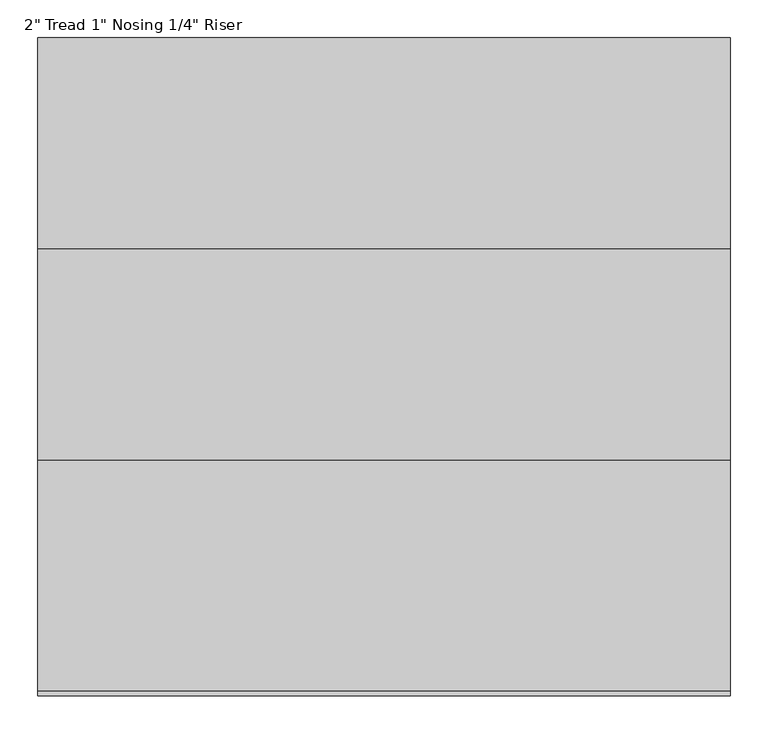
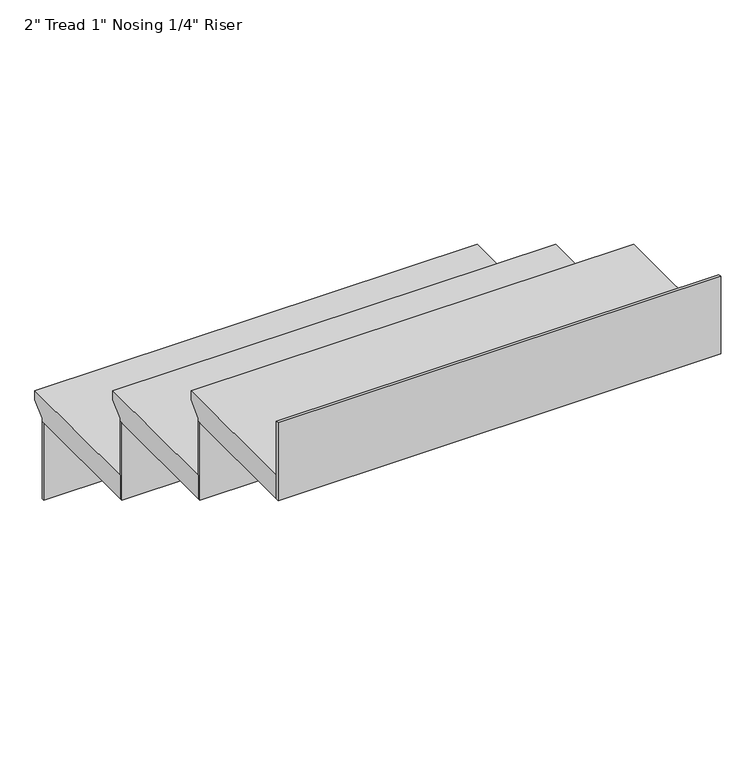
"""IFC4 building model written with IfcOpenShell, lengths in millimetres: stair flight geometry."""

from ifc_helpers import new_model, si_unit, frame, origin, place, context, project, spatial, polyline, outline, extrude, source, transform, mapped, element, save


def stair_flight_738362f5(model_context):
    return source(origin(), model_context, "Body", "SweptSolid", [
        extrude(outline(polyline([(-19826.9851539, 49110.6172466), (-19522.1851539, 49110.6172466), (-19522.1851539, 49091.5672466), (-19547.5851539, 49066.1672466), (-19547.5851539, 49059.8172466), (-19826.9851539, 49059.8172466), (-19826.9851539, 49110.6172466)])), frame((-2296.6415084, 0.0, 0.0), z_axis=(1.0, 0.0, 0.0), x_axis=(0.0, 1.0, 0.0)), (0.0, 0.0, 1.0), 914.4),
        extrude(outline(polyline([(-2296.6415084, -19553.9351539), (-2296.6415084, -19547.5851539), (-1382.2415084, -19547.5851539), (-1382.2415084, -19553.9351539), (-2296.6415084, -19553.9351539)])), frame((0.0, 0.0, 48890.4839133), z_axis=(0.0, 0.0, 1.0), x_axis=(1.0, 0.0, 0.0)), (0.0, 0.0, 1.0), 169.3333333),
        extrude(outline(polyline([(-2296.6415084, -19833.3351539), (-2296.6415084, -19826.9851539), (-1382.2415084, -19826.9851539), (-1382.2415084, -19833.3351539), (-2296.6415084, -19833.3351539)])), frame((0.0, 0.0, 49059.8172466), z_axis=(0.0, 0.0, 1.0), x_axis=(1.0, 0.0, 0.0)), (0.0, 0.0, 1.0), 169.3333333),
        extrude(outline(polyline([(-20106.3851539, 49279.9505799), (-19801.5851539, 49279.9505799), (-19801.5851539, 49260.9005799), (-19826.9851539, 49235.5005799), (-19826.9851539, 49229.1505799), (-20106.3851539, 49229.1505799), (-20106.3851539, 49279.9505799)])), frame((-2296.6415084, 0.0, 0.0), z_axis=(1.0, 0.0, 0.0), x_axis=(0.0, 1.0, 0.0)), (0.0, 0.0, 1.0), 914.4),
        extrude(outline(polyline([(-2296.6415084, -20112.7351539), (-2296.6415084, -20106.3851539), (-1382.2415084, -20106.3851539), (-1382.2415084, -20112.7351539), (-2296.6415084, -20112.7351539)])), frame((0.0, 0.0, 49229.1505799), z_axis=(0.0, 0.0, 1.0), x_axis=(1.0, 0.0, 0.0)), (0.0, 0.0, 1.0), 169.3333333),
        extrude(outline(polyline([(-2296.6415084, -20392.1351539), (-2296.6415084, -20385.7851539), (-1382.2415084, -20385.7851539), (-1382.2415084, -20392.1351539), (-2296.6415084, -20392.1351539)])), frame((0.0, 0.0, 49398.4839133), z_axis=(0.0, 0.0, 1.0), x_axis=(1.0, 0.0, 0.0)), (0.0, 0.0, 1.0), 169.3333333),
        extrude(outline(polyline([(-20385.7851539, 49449.2839133), (-20080.9851539, 49449.2839133), (-20080.9851539, 49430.2339133), (-20106.3851539, 49404.8339133), (-20106.3851539, 49398.4839133), (-20385.7851539, 49398.4839133), (-20385.7851539, 49449.2839133)])), frame((-2296.6415084, 0.0, 0.0), z_axis=(1.0, 0.0, 0.0), x_axis=(0.0, 1.0, 0.0)), (0.0, 0.0, 1.0), 914.4),
    ])


if __name__ == "__main__":
    model = new_model("IFC4")
    model_context = context("Model", 3, world=origin())
    ifc_project = project(units=[si_unit("LENGTHUNIT", "METRE", prefix="MILLI")], contexts=[model_context])
    site = spatial("IfcSite", under=ifc_project)
    building = spatial("IfcBuilding", under=site)
    placement = place(None, origin())
    stair_flight_shape = stair_flight_738362f5(model_context)
    element("IfcStairFlight", 1, ObjectType="2\" Tread 1\" Nosing 1/4\" Riser", at=placement, inside=building, context=model_context, shape_type="MappedRepresentation", body=[
        mapped(stair_flight_shape, transform((0.0, 0.0, 0.0), x_axis=(1.0, 0.0, 0.0), y_axis=(0.0, 1.0, 0.0), z_axis=(0.0, 0.0, 1.0))),
    ])
    save(model, "model.ifc")
